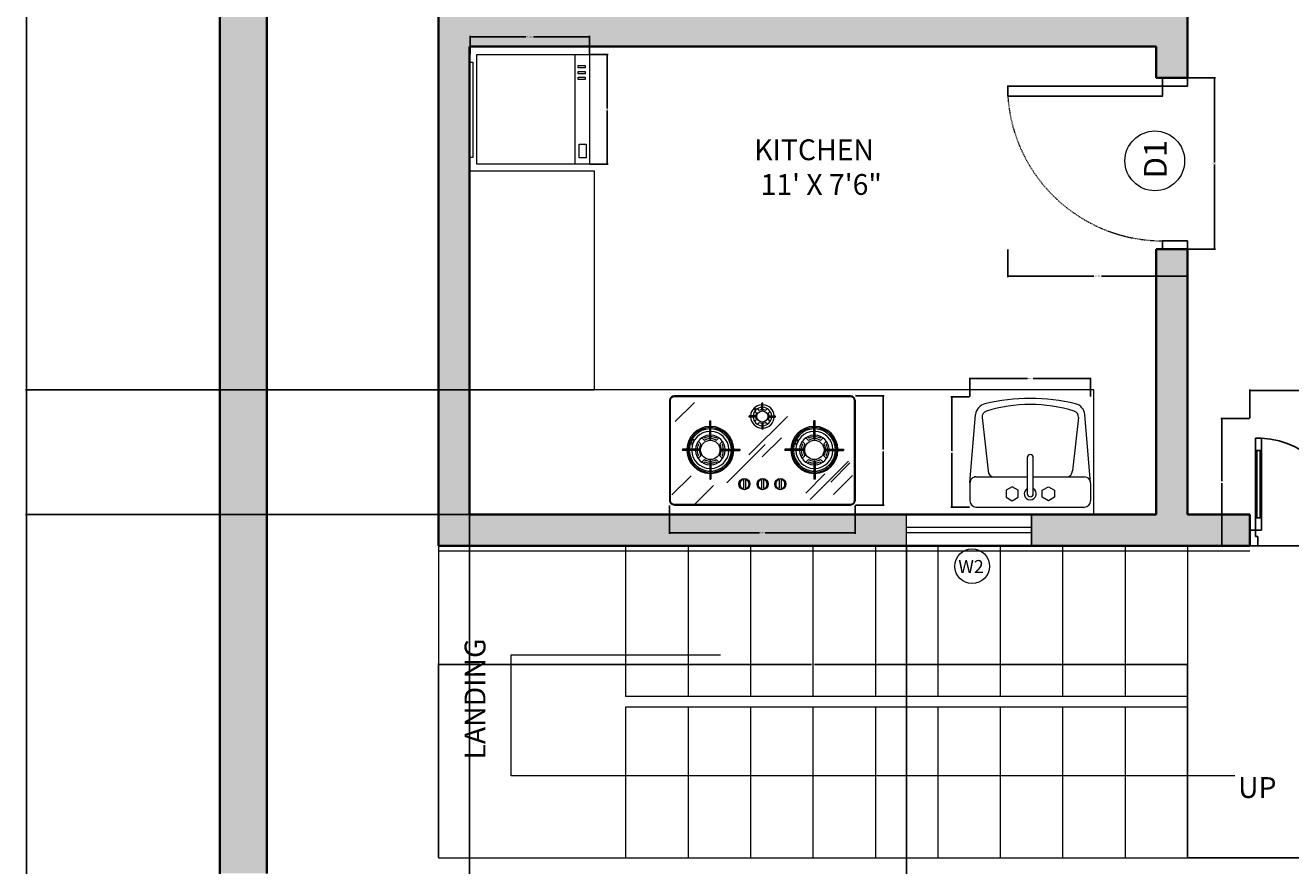
# Model space of a CAD drawing. Units: inches. Extents: x 2701 to 6846, y 811 to 2447.
# Tile 2 of 20: x 2701 to 2944, y 969 to 1130. Entities that reach past the tile are written whole.
import ezdxf

# ---------------------------------------------------------------- set-up
doc = ezdxf.new("R2010")
doc.units = ezdxf.units.IN
doc.linetypes.add('HIDDEN4', pattern=[0.09375, 0.0625, -0.03125])
for name, color, linetype, lineweight in [('A-ANNO-DIMS', 2, 'Continuous', 18), ('A-ANNO-IDEN', 7, 'Continuous', 13), ('A-ANNO-TEXT', 7, 'Continuous', 18), ('A-AREA-IDEN', 7, 'Continuous', 18), ('A-DOOR', 4, 'Continuous', 25), ('A-DOOR-SWNG', 4, 'HIDDEN4', 13), ('A-EQPM', 8, 'Continuous', 18), ('A-FLOR-FIXT', 7, 'Continuous', 18), ('A-FLOR-STRS', 7, 'Continuous', 18), ('A-GLAZ', 4, 'Continuous', 18), ('A-WALL', 7, 'Continuous', 35), ('C-PROP', 7, 'Continuous', 35)]:
    doc.layers.add(name, color=color, linetype=linetype, lineweight=lineweight)
doc.layers.add('A-WALL-PATT', color=18, linetype='Continuous', lineweight=13, true_color=0x000000)
doc.layers.add('C-PROP-PATT', color=18, linetype='Continuous', lineweight=13, true_color=0x000000)
doc.styles.get("Standard").update_dxf_attribs({"font": 'arial.ttf'})
doc.dimstyles.get("Standard").update_dxf_attribs({"dimtxt": 0.18, "dimasz": 0.18, "dimexe": 0.18, "dimexo": 0.0625, "dimgap": 0.09, "dimtad": 0, "dimtih": 1, "dimtoh": 1, "dimdec": 4, "dimzin": 0, "dimdsep": 46, "dimtxsty": 'Standard', "dimcen": 0.09, "dimadec": 0, "dimazin": 0, "dimtfac": 1, "dimtdec": 4, "dimtofl": 0, "dimtmove": 0, "dimatfit": 3, "dimfxl": 1, "dimtolj": 1, "dimtzin": 0, "dimarcsym": 0})

# ---------------------------------------------------------------- blocks, each defined once
blk = doc.blocks.new('A$C09A905BE')
for p, q in [((35, 690), (35, 610)), ((75, 690), (35, 690)), ((75, 610), (75, 690)), ((1125, 690), (1125, 610)), ((1165, 690), (1125, 690)), ((1165, 610), (1165, 690)), ((35, 610), (75, 610)), ((35, 180), (35, 610)), ((35, 610), (75, 610)), ((45, 180), (45, 610)), ((45, 610), (65, 610)), ((65, 610), (65, 180)), ((75, 610), (75, 180)), ((1125, 610), (1165, 610)), ((1125, 180), (1125, 610)), ((1125, 610), (1165, 610)), ((1135, 180), (1135, 610)), ((1135, 610), (1155, 610)), ((1155, 610), (1155, 180)), ((1165, 610), (1165, 180)), ((35, 100), (35, 180)), ((35, 180), (75, 180)), ((75, 180), (35, 180)), ((65, 180), (45, 180)), ((75, 180), (75, 100)), ((1125, 100), (1125, 180)), ((1125, 180), (1165, 180)), ((1165, 180), (1125, 180)), ((1155, 180), (1135, 180)), ((1165, 180), (1165, 100)), ((0, 0), (0, 100)), ((0, 100), (35, 100)), ((35, 100), (35, 60)), ((75, 100), (35, 100)), ((1165, 100), (1125, 100)), ((1165, 100), (1200, 100)), ((1165, 60), (1165, 100)), ((1200, 100), (1200, 0)), ((35, 60), (50, 60)), ((50, 60), (50, 50)), ((50, 50), (50, 0)), ((1150, 50), (1150, 60)), ((1150, 60), (1165, 60)), ((1150, 0), (1150, 50)), ((50, 0), (0, 0)), ((1200, 0), (1150, 0))]:
    blk.add_line(p, q)
for centre, start, end in [((42.5, 132.5), 356.66366, 86.66366), ((1157.5, 132.5), 93.33634, 183.33634)]:
    blk.add_arc(centre, 558.4, start, end)
blk = doc.blocks.new('MAIN DOOR')
blk.add_circle((3420.7, 1223.43), 3.42)
at = {"xscale": 0.03, "yscale": 0.03, "zscale": 0.03}
blk.add_blockref('A$C09A905BE', (3402.65, 1202.37), dxfattribs=at)
at = {"insert": (3418.39, 1224.62), "char_height": 2.5, "attachment_point": 1}
blk.add_mtext('MD', dxfattribs=at)
blk = doc.blocks.new('A$C301E58BA')
for p, q in [((0, 0.3491), (0, 0.4241)), ((0.475, 0.4491), (0.025, 0.4491)), ((0.15, 0.4085), (0.175, 0.423)), ((0.175, 0.423), (0.2, 0.4085)), ((0.325, 0.423), (0.3, 0.4085)), ((0.35, 0.4085), (0.325, 0.423)), ((0.5, 0.3491), (0.5, 0.4241)), ((0.15, 0.3797), (0.15, 0.4085)), ((0.175, 0.3652), (0.15, 0.3797)), ((0.2, 0.3797), (0.175, 0.3652)), ((0.2, 0.4085), (0.2, 0.3797)), ((0.2375, 0.3941), (0.2375, 0.2441)), ((0.2625, 0.2441), (0.2625, 0.3941)), ((0.3, 0.4085), (0.3, 0.3797)), ((0.3, 0.3797), (0.325, 0.3652)), ((0.325, 0.3652), (0.35, 0.3797)), ((0.35, 0.3797), (0.35, 0.4085)), ((0, 0.3491), (0.0236, 0.0657)), ((0.2375, 0.3241), (0.025, 0.3241)), ((0.475, 0.3241), (0.2625, 0.3241)), ((0.5, 0.3491), (0.4764, 0.0657)), ((0.0504, 0.0779), (0.075, 0.2991)), ((0.4496, 0.0779), (0.425, 0.2991))]:
    blk.add_line(p, q)
for centre, radius, start, end in [((0.025, 0.4241), 0.025, 90, 180), ((0.475, 0.4241), 0.025, 0, 90), ((0.25, 0.3941), 0.025, 300, 240), ((0.25, 0.3941), 0.0125, 0, 180), ((0.025, 0.3491), 0.025, 180, 270), ((0.1, 0.2991), 0.025, 90, 180), ((0.4, 0.2991), 0.025, 0, 90), ((0.475, 0.3491), 0.025, 270, 0), ((0.25, 0.2441), 0.0125, 180, 0), ((0.0734, 0.0698), 0.05, 184.7636, 256.6119), ((0.0753, 0.0751), 0.025, 173.6598, 253.0688), ((0.4247, 0.0751), 0.025, 286.9312, 6.3402), ((0.4266, 0.0698), 0.05, 283.3881, 355.2364), ((0.25, 0.8116), 0.8125, 256.6119, 283.3881), ((0.25, 0.6491), 0.625, 253.0688, 286.9312)]:
    blk.add_arc(centre, radius, start, end)
blk = doc.blocks.new('A$C038F079D')
for p, q in [((23.9, 336.8), (101.3, 414.2)), ((377.5, 410.6), (372.5, 410.6)), ((320.9, 202.7), (475.7, 357.5)), ((427.1, 359.8), (427.1, 354.8)), ((587.4, 339.9), (582.4, 339.9)), ((377.5, 305.6), (372.5, 305.6)), ((374.2, 193.8), (451.6, 271.2)), ((53.2, 224.7), (53.2, 219.7)), ((232.1, 89.3), (386.9, 244.1)), ((284, 224.7), (284, 219.7)), ((466, 224.7), (466, 219.7)), ((701.8, 224.7), (701.8, 219.7)), ((130.3, 173.3), (141.1, 184.1)), ((137.3, 169), (142.6, 174.2)), ((567.6, 22.2), (722.4, 177)), ((650.5, 92.2), (727.9, 169.6)), ((10.1, 41), (87.5, 118.4)), ((549.9, 47.9), (627.2, 125.3)), ((587.4, 103.7), (582.4, 103.7)), ((661.4, 42), (738.7, 119.3)), ((100.9, 1.5), (178.3, 78.9))]:
    blk.add_line(p, q)
at = {"ltscale": 0.18}
for p, q in [((372.5, 384.7), (372.5, 410.6)), ((377.5, 384.7), (377.5, 410.6)), ((322.3, 354.8), (322.3, 359.8)), ((347.6, 359.8), (322.3, 359.8)), ((350.8, 370.2), (343.5, 377.5)), ((362.2, 381.5), (354.8, 388.8)), ((387.8, 381.5), (395.2, 388.8)), ((399.2, 370.2), (406.5, 377.5)), ((402.4, 359.8), (427.1, 359.8)), ((162.6, 339.9), (167.6, 339.9)), ((162.6, 267.1), (162.6, 339.9)), ((167.6, 267.1), (167.6, 339.9)), ((347.6, 354.8), (322.3, 354.8)), ((343.5, 337.2), (350.8, 344.5)), ((354.8, 325.8), (362.2, 333.1)), ((372.5, 329.9), (372.5, 305.6)), ((377.5, 329.9), (377.5, 305.6)), ((395.2, 325.8), (387.8, 333.1)), ((406.5, 337.2), (399.2, 344.5)), ((402.4, 354.8), (427.1, 354.8)), ((582.4, 267.1), (582.4, 339.9)), ((587.4, 267.1), (587.4, 339.9)), ((116.2, 257), (127, 246.2)), ((130.3, 271.1), (141.1, 260.3)), ((137.3, 275.4), (142.6, 270.2)), ((187.6, 270.2), (192.8, 275.4)), ((189, 260.3), (199.8, 271.1)), ((203.2, 246.2), (214, 257)), ((546.8, 246.2), (536, 257)), ((561, 260.3), (550.2, 271.1)), ((562.4, 270.2), (557.2, 275.4)), ((612.7, 275.4), (607.4, 270.2)), ((619.7, 271.1), (608.9, 260.3)), ((633.8, 257), (623, 246.2)), ((125.1, 224.7), (53.2, 224.7)), ((125.1, 219.7), (53.2, 219.7)), ((111.9, 250), (117.1, 244.7)), ((210, 224.7), (284, 224.7)), ((210, 219.7), (284, 219.7)), ((213.1, 244.7), (218.3, 250)), ((540, 224.7), (466, 224.7)), ((540, 219.7), (466, 219.7)), ((536.9, 244.7), (531.7, 250)), ((629.9, 224.7), (701.8, 224.7)), ((629.9, 219.7), (701.8, 219.7)), ((638.1, 250), (632.9, 244.7)), ((111.9, 194.5), (117.1, 199.7)), ((116.2, 187.5), (127, 198.3)), ((162.6, 177.3), (162.6, 103.7)), ((167.6, 177.3), (167.6, 103.7)), ((187.6, 174.2), (192.8, 169)), ((189, 184.1), (199.8, 173.3)), ((203.2, 198.3), (214, 187.5)), ((213.1, 199.7), (218.3, 194.5)), ((536.9, 199.7), (531.7, 194.5)), ((546.8, 198.3), (536, 187.5)), ((561, 184.1), (550.2, 173.3)), ((562.4, 174.2), (557.2, 169)), ((582.4, 177.3), (582.4, 103.7)), ((587.4, 177.3), (587.4, 103.7)), ((612.7, 169), (607.4, 174.2)), ((619.7, 173.3), (608.9, 184.1)), ((633.8, 187.5), (623, 198.3)), ((638.1, 194.5), (632.9, 199.7)), ((162.6, 103.7), (167.6, 103.7)), ((298.6, 99.8), (298.6, 69)), ((306.6, 99.8), (306.6, 69)), ((372, 99.8), (372, 69)), ((380, 99.8), (380, 69)), ((443.4, 99.8), (443.4, 69)), ((451.4, 99.8), (451.4, 69))]:
    blk.add_line(p, q, dxfattribs=at)
for points in [[(20, 0), (730, 0, 0.414214), (750, 20), (750, 420, 0.414214), (730, 440), (20, 440, 0.414214), (0, 420), (0, 20, 0.414214)], [(20, 3), (730, 3, 0.414214), (747, 20), (747, 420, 0.414214), (730, 437), (20, 437, 0.414214), (3, 420), (3, 20, 0.414214)]]:
    blk.add_lwpolyline(points, format="xyb", close=True)
for centre in [(345.9, 386.3), (94.7, 261.5), (514.6, 260.8), (89.1, 248.3), (509, 247.6)]:
    blk.add_circle(centre, 3.73)
for centre, radius in [((375, 357.3), 22.4), ((165.1, 222.2), 39), ((584.9, 222.2), 39), ((302.6, 84.4), 22.5), ((302.6, 84.4), 21.5), ((376, 84.4), 22.5), ((376, 84.4), 21.5), ((447.4, 84.4), 22.5), ((447.4, 84.4), 21.5)]:
    blk.add_circle(centre, radius, dxfattribs=at)
for centre, radius, start, end in [((375, 357.3), 47.4, 93.0255, 176.9745), ((375, 357.3), 37.4, 93.8363, 176.1637), ((346.8, 357.3), 2.62, 287.6318, 72.3682), ((375, 357.3), 27.4, 151.9979, 174.8384), ((375, 357.3), 27.4, 95.203, 118.0021), ((375, 385), 2.52, 187.9505, 352.0495), ((375, 357.3), 47.4, 3.0255, 86.9745), ((375, 357.3), 37.4, 3.8363, 86.1637), ((375, 357.3), 27.4, 61.9979, 84.797), ((375, 357.3), 27.4, 5.206, 28.0021), ((402.7, 357.3), 2.52, 97.2236, 262.7764), ((165.1, 222.2), 95, 91.5918, 178.4082), ((165.1, 222.2), 90, 91.5918, 178.4082), ((165.1, 222.2), 85, 91.6854, 178.3146), ((165.1, 222.2), 90, 1.5918, 88.4082), ((165.1, 222.2), 85, 1.6854, 88.3146), ((165.1, 222.2), 95, 1.5918, 88.4082), ((375, 357.3), 47.4, 183.0255, 266.9745), ((375, 357.3), 37.4, 183.8363, 266.1637), ((375, 357.3), 27.4, 185.1616, 208.0021), ((375, 357.3), 27.4, 241.9979, 264.7569), ((375, 330), 2.5, 358.3317, 181.6683), ((375, 357.3), 47.4, 273.0255, 356.9745), ((375, 357.3), 37.4, 273.8363, 356.1637), ((375, 357.3), 27.4, 275.2431, 298.0021), ((375, 357.3), 27.4, 331.9979, 354.794), ((584.9, 222.2), 95, 91.5918, 178.4082), ((584.9, 222.2), 90, 91.5918, 178.4082), ((584.9, 222.2), 85, 91.6854, 178.3146), ((584.9, 222.2), 90, 1.5918, 88.4082), ((584.9, 222.2), 85, 1.6854, 88.3146), ((584.9, 222.2), 95, 1.5918, 88.4082), ((165.1, 222.2), 75, 91.9102, 178.0898), ((165.1, 222.2), 60, 92.388, 177.612), ((165.1, 222.2), 45, 93.1847, 122.1604), ((165.1, 222.2), 53, 92.7036, 115.1461), ((165.1, 267.4), 2.52, 186.7354, 353.2646), ((165.1, 222.2), 75, 1.9102, 88.0898), ((165.1, 222.2), 60, 2.388, 87.612), ((165.1, 222.2), 53, 64.8539, 87.2964), ((165.1, 222.2), 45, 57.8396, 86.8153), ((584.9, 222.2), 75, 91.9102, 178.0898), ((584.9, 222.2), 60, 92.388, 177.612), ((584.9, 222.2), 45, 93.1847, 122.1604), ((584.9, 222.2), 53, 92.7036, 115.1461), ((584.9, 267.3), 2.51, 183.9579, 356.0421), ((584.9, 222.2), 75, 1.9102, 88.0898), ((584.9, 222.2), 60, 2.388, 87.612), ((584.9, 222.2), 53, 64.8539, 87.2964), ((584.9, 222.2), 45, 57.8396, 86.8153), ((165.1, 222.2), 95, 181.5918, 268.4082), ((165.1, 222.2), 90, 181.5918, 268.4082), ((165.1, 222.2), 85, 181.6854, 268.3146), ((165.1, 222.2), 75, 181.9102, 268.0898), ((165.1, 222.2), 60, 182.388, 267.612), ((165.1, 222.2), 53, 154.8539, 177.2964), ((165.1, 222.2), 53, 182.7036, 205.1461), ((165.1, 222.2), 45, 147.8396, 176.8153), ((119.3, 222.2), 2.64, 288.751, 71.249), ((165.1, 222.2), 45, 183.1847, 212.1604), ((165.1, 222.2), 75, 271.9102, 358.0898), ((165.1, 222.2), 60, 272.388, 357.612), ((165.1, 222.2), 85, 271.6854, 358.3146), ((165.1, 222.2), 90, 271.5918, 358.4082), ((165.1, 222.2), 95, 271.5918, 358.4082), ((165.1, 222.2), 45, 3.1847, 32.1604), ((165.1, 222.2), 45, 327.8396, 356.8153), ((210.9, 222.2), 2.67, 110.5507, 249.4493), ((165.1, 222.2), 53, 2.7036, 25.1461), ((165.1, 222.2), 53, 334.8539, 357.2964), ((584.9, 222.2), 95, 181.5918, 268.4082), ((584.9, 222.2), 90, 181.5918, 268.4082), ((584.9, 222.2), 85, 181.6854, 268.3146), ((584.9, 222.2), 75, 181.9102, 268.0898), ((584.9, 222.2), 60, 182.388, 267.612), ((584.9, 222.2), 53, 154.8539, 177.2964), ((584.9, 222.2), 53, 182.7036, 205.1461), ((584.9, 222.2), 45, 147.8396, 176.8153), ((539.2, 222.2), 2.63, 288.412, 71.588), ((584.9, 222.2), 45, 183.1847, 212.1604), ((584.9, 222.2), 90, 271.5918, 358.4082), ((584.9, 222.2), 85, 271.6854, 358.3146), ((584.9, 222.2), 75, 271.9102, 358.0898), ((584.9, 222.2), 60, 272.388, 357.612), ((584.9, 222.2), 95, 271.5918, 358.4082), ((584.9, 222.2), 45, 3.1847, 32.1604), ((584.9, 222.2), 45, 327.8396, 356.8153), ((630.5, 222.2), 2.58, 104.2945, 255.7055), ((584.9, 222.2), 53, 2.7036, 25.1461), ((584.9, 222.2), 53, 334.8539, 357.2964), ((165.1, 222.2), 45, 237.8396, 266.8153), ((165.1, 222.2), 53, 244.8539, 267.2964), ((165.1, 222.2), 45, 273.1847, 302.1604), ((165.1, 222.2), 53, 272.7036, 295.1461), ((584.9, 222.2), 45, 237.8396, 266.8153), ((584.9, 222.2), 53, 244.8539, 267.2964), ((584.9, 176.5), 2.63, 17.9418, 162.0582), ((584.9, 222.2), 45, 273.1847, 302.1604), ((584.9, 222.2), 53, 272.7036, 295.1461), ((302.6, 84.4), 18.5, 111.3237, 248.6763), ((296.6, 99.8), 2, 0, 111.3237), ((296.6, 69), 2, 248.6763, 0), ((308.6, 99.8), 2, 68.6763, 180), ((308.6, 69), 2, 180, 291.3237), ((302.6, 84.4), 18.5, 291.3237, 68.6763), ((376, 84.4), 18.5, 111.3237, 248.6763), ((370, 99.8), 2, 0, 111.3237), ((370, 69), 2, 248.6763, 0), ((382, 99.8), 2, 68.6763, 180), ((382, 69), 2, 180, 291.3237), ((376, 84.4), 18.5, 291.3237, 68.6763), ((447.4, 84.4), 18.5, 111.3237, 248.6763), ((441.4, 99.8), 2, 0, 111.3237), ((441.4, 69), 2, 248.6763, 0), ((453.4, 99.8), 2, 68.6763, 180), ((453.4, 69), 2, 180, 291.3237), ((447.4, 84.4), 18.5, 291.3237, 68.6763)]:
    blk.add_arc(centre, radius, start, end, dxfattribs=at)
blk.add_arc((165.1, 176.3), 2.69, 21.7885, 158.2115)
blk = doc.blocks.new('A$C45054F6D')
for p, q in [((33.6, 610), (522.2, 610)), ((33.6, 596), (33.6, 610)), ((522.2, 596), (33.6, 596)), ((522.2, 610), (522.2, 596)), ((0, 575.1), (560, 575.1)), ((0, 0), (0, 575.1)), ((560, 575.1), (560, 0)), ((560, 75), (0, 75)), ((33.3, 53), (103.3, 53)), ((33.3, 16.3), (33.3, 53)), ((103.3, 16.3), (33.3, 16.3)), ((103.3, 53), (103.3, 16.3)), ((432.3, 21.5), (432.3, 58.3)), ((432.3, 58.3), (444.6, 58.3)), ((444.6, 21.5), (432.3, 21.5)), ((444.6, 58.3), (444.6, 21.5)), ((462.1, 21.5), (462.1, 58.3)), ((462.1, 58.3), (474.3, 58.3)), ((474.3, 21.5), (462.1, 21.5)), ((474.3, 58.3), (474.3, 21.5)), ((491.8, 21.5), (491.8, 58.3)), ((491.8, 58.3), (504.1, 58.3)), ((504.1, 21.5), (491.8, 21.5)), ((504.1, 58.3), (504.1, 21.5)), ((560, 0), (0, 0))]:
    blk.add_line(p, q)
blk = doc.blocks.new('DOOR-D1-33IN-PANEL-FRAME')
blk.add_lwpolyline([(0, 33), (0, 31.37), (4.8, 31.37), (4.8, 33), (0, 33)], close=True)
for points in [[(4.32, 33), (0.48, 33)], [(4.8, 0), (4.8, 3.55), (34.54, 3.55), (34.54, 1.63), (0, 1.63), (0, 0)], [(0, 0), (4.8, 0)], [(4.32, 0), (0.48, 0)]]:
    blk.add_lwpolyline(points)
blk = doc.blocks.new('WIN-W2-24IN')
for p, q in [((24, 6), (0, 6)), ((24, 6), (0, 6)), ((0, 0), (0, 6)), ((24, 6), (24, 6)), ((24, 6), (24, 0)), ((24, 3.5), (0, 3.5)), ((24, 2.5), (0, 2.5)), ((24, 0), (0, 0))]:
    blk.add_line(p, q)
blk = doc.blocks.new('*D27')
at = {"layer": 'A-ANNO-DIMS', "color": 0, "lineweight": -2, "transparency": 16777216}
for p, q in [((2889.43, 1086.99), (2889.43, 1081.69)), ((2923.97, 1086.99), (2923.97, 1081.69)), ((2889.61, 1081.87), (2905.98, 1081.87)), ((2923.79, 1081.87), (2907.42, 1081.87))]:
    blk.add_line(p, q, dxfattribs=at)
at = {"layer": 'A-ANNO-DIMS', "color": 0, "transparency": 16777216}
for points in [[(2889.61, 1081.9), (2889.61, 1081.84), (2889.43, 1081.87)], [(2923.79, 1081.9), (2923.79, 1081.84), (2923.97, 1081.87)]]:
    blk.add_solid(points, dxfattribs=at)
at = {"layer": 'Defpoints', "color": 0, "transparency": 16777216}
for p in [(2889.43, 1087.05), (2923.97, 1087.05), (2889.43, 1081.87)]:
    blk.add_point(p, dxfattribs=at)
at = {"layer": 'A-ANNO-DIMS', "color": 0, "transparency": 16777216, "insert": (2906.7, 1081.87), "char_height": 0.18, "attachment_point": 5}
blk.add_mtext('\\A1;D1 35 TYP.', dxfattribs=at)
blk = doc.blocks.new('*D28')
at = {"layer": 'A-ANNO-DIMS', "color": 0, "lineweight": -2, "transparency": 16777216}
for p, q in [((2924.03, 1120.05), (2929.33, 1120.05)), ((2929.15, 1119.87), (2929.15, 1103.73)), ((2929.15, 1087.23), (2929.15, 1103.37)), ((2924.03, 1087.05), (2929.33, 1087.05))]:
    blk.add_line(p, q, dxfattribs=at)
at = {"layer": 'A-ANNO-DIMS', "color": 0, "transparency": 16777216}
for points in [[(2929.12, 1119.87), (2929.18, 1119.87), (2929.15, 1120.05)], [(2929.12, 1087.23), (2929.18, 1087.23), (2929.15, 1087.05)]]:
    blk.add_solid(points, dxfattribs=at)
at = {"layer": 'Defpoints', "color": 0, "transparency": 16777216}
for p in [(2923.97, 1120.05), (2923.97, 1087.05), (2929.15, 1087.05)]:
    blk.add_point(p, dxfattribs=at)
at = {"layer": 'A-ANNO-DIMS', "color": 0, "transparency": 16777216, "insert": (2929.15, 1103.55), "char_height": 0.18, "attachment_point": 5}
blk.add_mtext('\\A1;33 TYP.', dxfattribs=at)
blk = doc.blocks.new('*D31')
at = {"layer": 'A-ANNO-DIMS', "color": 0, "lineweight": -2, "transparency": 16777216}
for p, q in [((2935.97, 1054.6), (2935.97, 1060.11)), ((2936.15, 1059.93), (2952.88, 1059.93)), ((2971.79, 1059.93), (2955.06, 1059.93)), ((2971.97, 1054.6), (2971.97, 1060.11))]:
    blk.add_line(p, q, dxfattribs=at)
at = {"layer": 'A-ANNO-DIMS', "color": 0, "transparency": 16777216}
for points in [[(2936.15, 1059.96), (2936.15, 1059.9), (2935.97, 1059.93)], [(2971.79, 1059.96), (2971.79, 1059.9), (2971.97, 1059.93)]]:
    blk.add_solid(points, dxfattribs=at)
at = {"layer": 'Defpoints', "color": 0, "transparency": 16777216}
for p in [(2971.97, 1059.93), (2935.97, 1054.53), (2971.97, 1054.53)]:
    blk.add_point(p, dxfattribs=at)
at = {"layer": 'A-ANNO-DIMS', "color": 0, "transparency": 16777216, "insert": (2953.97, 1059.93), "char_height": 0.18, "attachment_point": 5}
blk.add_mtext('\\A1;ENTRY DOOR 36', dxfattribs=at)
blk = doc.blocks.new('*D32')
at = {"layer": 'A-ANNO-DIMS', "color": 0, "lineweight": -2, "transparency": 16777216}
for p, q in [((2935.91, 1054.53), (2930.39, 1054.53)), ((2930.57, 1054.35), (2930.57, 1042.47)), ((2930.57, 1030.23), (2930.57, 1042.11)), ((2935.91, 1030.05), (2930.39, 1030.05))]:
    blk.add_line(p, q, dxfattribs=at)
at = {"layer": 'A-ANNO-DIMS', "color": 0, "transparency": 16777216}
for points in [[(2930.54, 1054.35), (2930.6, 1054.35), (2930.57, 1054.53)], [(2930.54, 1030.23), (2930.6, 1030.23), (2930.57, 1030.05)]]:
    blk.add_solid(points, dxfattribs=at)
at = {"layer": 'Defpoints', "color": 0, "transparency": 16777216}
for p in [(2930.57, 1054.53), (2935.97, 1054.53), (2935.97, 1030.05)]:
    blk.add_point(p, dxfattribs=at)
at = {"layer": 'A-ANNO-DIMS', "color": 0, "transparency": 16777216, "insert": (2930.57, 1042.29), "char_height": 0.18, "attachment_point": 5}
blk.add_mtext('\\A1;24', dxfattribs=at)
blk = doc.blocks.new('*D55')
at = {"layer": 'A-ANNO-DIMS', "color": 0, "lineweight": -2, "transparency": 16777216}
for p, q in [((2882.15, 1058.77), (2882.15, 1062.37)), ((2882.33, 1062.19), (2893.2, 1062.19)), ((2905.16, 1062.19), (2894.29, 1062.19)), ((2905.34, 1058.77), (2905.34, 1062.37))]:
    blk.add_line(p, q, dxfattribs=at)
at = {"layer": 'A-ANNO-DIMS', "color": 0, "transparency": 16777216}
for points in [[(2882.33, 1062.22), (2882.33, 1062.16), (2882.15, 1062.19)], [(2905.16, 1062.22), (2905.16, 1062.16), (2905.34, 1062.19)]]:
    blk.add_solid(points, dxfattribs=at)
at = {"layer": 'Defpoints', "color": 0, "transparency": 16777216}
for p in [(2882.15, 1062.19), (2882.15, 1058.71), (2905.34, 1058.71)]:
    blk.add_point(p, dxfattribs=at)
at = {"layer": 'A-ANNO-DIMS', "color": 0, "transparency": 16777216, "insert": (2893.74, 1062.19), "char_height": 0.18, "attachment_point": 5}
blk.add_mtext('\\A1;SINK 23', dxfattribs=at)
blk = doc.blocks.new('*D56')
at = {"layer": 'A-ANNO-DIMS', "color": 0, "lineweight": -2, "transparency": 16777216}
for p, q in [((2882.09, 1058.71), (2878.5, 1058.71)), ((2878.68, 1058.53), (2878.68, 1048.29)), ((2878.68, 1037.68), (2878.68, 1047.93)), ((2882.09, 1037.5), (2878.5, 1037.5))]:
    blk.add_line(p, q, dxfattribs=at)
at = {"layer": 'A-ANNO-DIMS', "color": 0, "transparency": 16777216}
for points in [[(2878.65, 1058.53), (2878.71, 1058.53), (2878.68, 1058.71)], [(2878.65, 1037.68), (2878.71, 1037.68), (2878.68, 1037.5)]]:
    blk.add_solid(points, dxfattribs=at)
at = {"layer": 'Defpoints', "color": 0, "transparency": 16777216}
for p in [(2882.15, 1058.71), (2878.68, 1037.5), (2882.15, 1037.5)]:
    blk.add_point(p, dxfattribs=at)
at = {"layer": 'A-ANNO-DIMS', "color": 0, "transparency": 16777216, "insert": (2878.68, 1048.11), "char_height": 0.18, "attachment_point": 5}
blk.add_mtext('\\A1;21', dxfattribs=at)
blk = doc.blocks.new('*D57')
at = {"layer": 'A-ANNO-DIMS', "color": 0, "lineweight": -2, "transparency": 16777216}
for p, q in [((2824.38, 1037.83), (2824.38, 1032.35)), ((2860.12, 1037.83), (2860.12, 1032.35)), ((2824.56, 1032.53), (2841.73, 1032.53)), ((2859.94, 1032.53), (2842.77, 1032.53))]:
    blk.add_line(p, q, dxfattribs=at)
at = {"layer": 'A-ANNO-DIMS', "color": 0, "transparency": 16777216}
for points in [[(2824.56, 1032.56), (2824.56, 1032.5), (2824.38, 1032.53)], [(2859.94, 1032.56), (2859.94, 1032.5), (2860.12, 1032.53)]]:
    blk.add_solid(points, dxfattribs=at)
at = {"layer": 'Defpoints', "color": 0, "transparency": 16777216}
for p in [(2824.38, 1037.89), (2860.12, 1037.89), (2860.12, 1032.53)]:
    blk.add_point(p, dxfattribs=at)
at = {"layer": 'A-ANNO-DIMS', "color": 0, "transparency": 16777216, "insert": (2842.25, 1032.53), "char_height": 0.18, "attachment_point": 5}
blk.add_mtext('\\A1;HOB 36', dxfattribs=at)
blk = doc.blocks.new('*D58')
at = {"layer": 'A-ANNO-DIMS', "color": 0, "lineweight": -2, "transparency": 16777216}
for p, q in [((2860.18, 1058.86), (2865.66, 1058.86)), ((2865.48, 1058.68), (2865.48, 1048.55)), ((2865.48, 1038.07), (2865.48, 1048.19)), ((2860.18, 1037.89), (2865.66, 1037.89))]:
    blk.add_line(p, q, dxfattribs=at)
at = {"layer": 'A-ANNO-DIMS', "color": 0, "transparency": 16777216}
for points in [[(2865.45, 1058.68), (2865.51, 1058.68), (2865.48, 1058.86)], [(2865.45, 1038.07), (2865.51, 1038.07), (2865.48, 1037.89)]]:
    blk.add_solid(points, dxfattribs=at)
at = {"layer": 'Defpoints', "color": 0, "transparency": 16777216}
for p in [(2860.12, 1058.86), (2865.48, 1058.86), (2860.12, 1037.89)]:
    blk.add_point(p, dxfattribs=at)
at = {"layer": 'A-ANNO-DIMS', "color": 0, "transparency": 16777216, "insert": (2865.48, 1048.37), "char_height": 0.18, "attachment_point": 5}
blk.add_mtext('\\A1;21', dxfattribs=at)
blk = doc.blocks.new('*D59')
at = {"layer": 'A-ANNO-DIMS', "color": 0, "lineweight": -2, "transparency": 16777216}
for p, q in [((2786.06, 1124.54), (2786.06, 1128.1)), ((2786.24, 1127.92), (2796.81, 1127.92)), ((2808.83, 1127.92), (2798.26, 1127.92)), ((2809.01, 1124.54), (2809.01, 1128.1))]:
    blk.add_line(p, q, dxfattribs=at)
at = {"layer": 'A-ANNO-DIMS', "color": 0, "transparency": 16777216}
for points in [[(2786.24, 1127.95), (2786.24, 1127.89), (2786.06, 1127.92)], [(2808.83, 1127.95), (2808.83, 1127.89), (2809.01, 1127.92)]]:
    blk.add_solid(points, dxfattribs=at)
at = {"layer": 'Defpoints', "color": 0, "transparency": 16777216}
for p in [(2786.06, 1127.92), (2786.06, 1124.48), (2809.01, 1124.48)]:
    blk.add_point(p, dxfattribs=at)
at = {"layer": 'A-ANNO-DIMS', "color": 0, "transparency": 16777216, "insert": (2797.53, 1127.92), "char_height": 0.18, "attachment_point": 5}
blk.add_mtext('\\A1;FRIDGE 23', dxfattribs=at)
blk = doc.blocks.new('*D60')
at = {"layer": 'A-ANNO-DIMS', "color": 0, "lineweight": -2, "transparency": 16777216}
for p, q in [((2809.07, 1124.48), (2812.63, 1124.48)), ((2812.45, 1124.3), (2812.45, 1114.12)), ((2812.45, 1103.59), (2812.45, 1113.76)), ((2809.07, 1103.41), (2812.63, 1103.41))]:
    blk.add_line(p, q, dxfattribs=at)
at = {"layer": 'A-ANNO-DIMS', "color": 0, "transparency": 16777216}
for points in [[(2812.42, 1124.3), (2812.48, 1124.3), (2812.45, 1124.48)], [(2812.42, 1103.59), (2812.48, 1103.59), (2812.45, 1103.41)]]:
    blk.add_solid(points, dxfattribs=at)
at = {"layer": 'Defpoints', "color": 0, "transparency": 16777216}
for p in [(2809.01, 1124.48), (2812.45, 1124.48), (2809.01, 1103.41)]:
    blk.add_point(p, dxfattribs=at)
at = {"layer": 'A-ANNO-DIMS', "color": 0, "transparency": 16777216, "insert": (2812.45, 1113.94), "char_height": 0.18, "attachment_point": 5}
blk.add_mtext('\\A1;21', dxfattribs=at)
blk = doc.blocks.new('*D66')
at = {"layer": 'A-ANNO-DIMS', "color": 0, "lineweight": -2, "transparency": 16777216}
for p, q in [((2737.91, 1504.05), (2700.59, 1504.05)), ((2700.77, 1503.87), (2700.77, 1180.23)), ((2700.77, 856.23), (2700.77, 1179.87)), ((2737.91, 856.05), (2700.59, 856.05))]:
    blk.add_line(p, q, dxfattribs=at)
at = {"layer": 'A-ANNO-DIMS', "color": 0, "transparency": 16777216}
for points in [[(2700.74, 1503.87), (2700.8, 1503.87), (2700.77, 1504.05)], [(2700.74, 856.23), (2700.8, 856.23), (2700.77, 856.05)]]:
    blk.add_solid(points, dxfattribs=at)
at = {"layer": 'Defpoints', "color": 0, "transparency": 16777216}
for p in [(2700.77, 1504.05), (2737.97, 1504.05), (2737.97, 856.05)]:
    blk.add_point(p, dxfattribs=at)
at = {"layer": 'A-ANNO-DIMS', "color": 0, "transparency": 16777216, "insert": (2700.77, 1180.05), "char_height": 0.18, "attachment_point": 5}
blk.add_mtext('\\A1;648', dxfattribs=at)
blk = doc.blocks.new('*D73')
at = {"layer": 'A-ANNO-DIMS', "color": 0, "lineweight": -2, "transparency": 16777216}
for p, q in [((2809.91, 1060.05), (2700.59, 1060.05)), ((2700.77, 1059.87), (2700.77, 1048.23)), ((2700.77, 1036.23), (2700.77, 1047.87)), ((2785.91, 1036.05), (2700.59, 1036.05))]:
    blk.add_line(p, q, dxfattribs=at)
at = {"layer": 'A-ANNO-DIMS', "color": 0, "transparency": 16777216}
for points in [[(2700.74, 1059.87), (2700.8, 1059.87), (2700.77, 1060.05)], [(2700.74, 1036.23), (2700.8, 1036.23), (2700.77, 1036.05)]]:
    blk.add_solid(points, dxfattribs=at)
at = {"layer": 'Defpoints', "color": 0, "transparency": 16777216}
for p in [(2700.77, 1060.05), (2809.97, 1060.05), (2785.97, 1036.05)]:
    blk.add_point(p, dxfattribs=at)
at = {"layer": 'A-ANNO-DIMS', "color": 0, "transparency": 16777216, "insert": (2700.77, 1048.05), "char_height": 0.18, "attachment_point": 5}
blk.add_mtext('\\A1;24', dxfattribs=at)
blk = doc.blocks.new('*D74')
at = {"layer": 'A-ANNO-DIMS', "color": 0, "lineweight": -2, "transparency": 16777216}
for p, q in [((2785.97, 1035.99), (2785.97, 818.67)), ((2869.97, 1029.99), (2869.97, 818.67)), ((2786.15, 818.85), (2827.75, 818.85)), ((2869.79, 818.85), (2828.19, 818.85))]:
    blk.add_line(p, q, dxfattribs=at)
at = {"layer": 'A-ANNO-DIMS', "color": 0, "transparency": 16777216}
for points in [[(2786.15, 818.88), (2786.15, 818.82), (2785.97, 818.85)], [(2869.79, 818.88), (2869.79, 818.82), (2869.97, 818.85)]]:
    blk.add_solid(points, dxfattribs=at)
at = {"layer": 'Defpoints', "color": 0, "transparency": 16777216}
for p in [(2785.97, 1036.05), (2869.97, 1030.05), (2869.97, 818.85)]:
    blk.add_point(p, dxfattribs=at)
at = {"layer": 'A-ANNO-DIMS', "color": 0, "transparency": 16777216, "insert": (2827.97, 818.85), "char_height": 0.18, "attachment_point": 5}
blk.add_mtext('\\A1;84', dxfattribs=at)
blk = doc.blocks.new('*D78')
at = {"layer": 'A-ANNO-DIMS', "color": 0, "lineweight": -2, "transparency": 16777216}
for p, q in [((2779.97, 970.11), (2779.97, 1007.43)), ((2780.15, 1007.25), (2851.69, 1007.25)), ((2923.79, 1007.25), (2852.25, 1007.25)), ((2923.97, 970.11), (2923.97, 1007.43))]:
    blk.add_line(p, q, dxfattribs=at)
at = {"layer": 'A-ANNO-DIMS', "color": 0, "transparency": 16777216}
for points in [[(2780.15, 1007.28), (2780.15, 1007.22), (2779.97, 1007.25)], [(2923.79, 1007.28), (2923.79, 1007.22), (2923.97, 1007.25)]]:
    blk.add_solid(points, dxfattribs=at)
at = {"layer": 'Defpoints', "color": 0, "transparency": 16777216}
for p in [(2923.97, 1007.25), (2779.97, 970.05), (2923.97, 970.05)]:
    blk.add_point(p, dxfattribs=at)
at = {"layer": 'A-ANNO-DIMS', "color": 0, "transparency": 16777216, "insert": (2851.97, 1007.25), "char_height": 0.18, "attachment_point": 5}
blk.add_mtext('\\A1;144', dxfattribs=at)
blk = doc.blocks.new('*D79')
at = {"layer": 'A-ANNO-DIMS', "color": 0, "lineweight": -2, "transparency": 16777216}
for p, q in [((2924.03, 1030.05), (2961.35, 1030.05)), ((2961.17, 1029.87), (2961.17, 1000.23)), ((2961.17, 970.23), (2961.17, 999.87)), ((2924.03, 970.05), (2961.35, 970.05))]:
    blk.add_line(p, q, dxfattribs=at)
at = {"layer": 'A-ANNO-DIMS', "color": 0, "transparency": 16777216}
for points in [[(2961.14, 1029.87), (2961.2, 1029.87), (2961.17, 1030.05)], [(2961.14, 970.23), (2961.2, 970.23), (2961.17, 970.05)]]:
    blk.add_solid(points, dxfattribs=at)
at = {"layer": 'Defpoints', "color": 0, "transparency": 16777216}
for p in [(2923.97, 1030.05), (2923.97, 970.05), (2961.17, 970.05)]:
    blk.add_point(p, dxfattribs=at)
at = {"layer": 'A-ANNO-DIMS', "color": 0, "transparency": 16777216, "insert": (2961.17, 1000.05), "char_height": 0.18, "attachment_point": 5}
blk.add_mtext('\\A1;60', dxfattribs=at)

msp = doc.modelspace()

# ---------------------------------------------------------------- hatches: boundary and pattern name
at = {"layer": 'A-WALL-PATT'}
h = msp.add_hatch(color=256, dxfattribs=at)
h.dxf.hatch_style = 1
h.paths.add_polyline_path([(3085.97, 1456.05), (3085.97, 1348.05), (3091.97, 1348.05), (3091.97, 1360.05), (3091.97, 1462.05), (2960.09, 1462.05), (2960.09, 1456.05), (2971.97, 1456.05), (2971.97, 1372.05), (2923.97, 1372.05), (2923.97, 1378.05), (2917.97, 1378.05), (2917.97, 1351.05), (2923.97, 1351.05), (2923.97, 1366.05), (2971.97, 1366.05), (2971.97, 1351.05), (2976.77, 1351.05), (2977.97, 1351.05), (2977.97, 1456.05)])
h.paths.add_polyline_path([(2779.97, 1462.05), (2779.97, 1342.05), (2785.97, 1342.05), (2785.97, 1456.05), (2917.97, 1456.05), (2917.97, 1408.05), (2922.33, 1408.05), (2923.97, 1408.05), (2923.97, 1456.05), (2937.09, 1456.05), (2937.09, 1462.05)])
h.paths.add_polyline_path([(2779.97, 1306.05), (2779.97, 1294.24), (2785.97, 1294.24), (2785.97, 1306.05), (2851.37, 1306.05, -0.025815), (2852.62, 1306.11, -0.025815), (2853.87, 1306.05), (2863.97, 1306.05), (2863.97, 1258.05), (2857.97, 1258.05), (2857.97, 1252.05), (2878.97, 1252.05), (2878.97, 1258.05), (2869.97, 1258.05), (2869.97, 1306.05), (2923.97, 1306.05), (2923.97, 1318.05), (2919.17, 1318.05), (2917.97, 1318.05), (2917.97, 1312.05), (2785.97, 1312.05), (2785.97, 1318.05), (2779.97, 1318.05)])
h.paths.add_polyline_path([(2785.97, 1252.05), (2827.97, 1252.05), (2827.97, 1256.41), (2827.97, 1258.05), (2785.97, 1258.05), (2785.97, 1271.24), (2779.97, 1271.24), (2779.97, 1174.05), (2785.97, 1174.05)])
h.paths.add_polyline_path([(2779.97, 1030.05), (2869.97, 1030.05), (2869.97, 1036.05), (2785.97, 1036.05), (2785.97, 1126.05), (2917.97, 1126.05), (2917.97, 1120.05), (2923.97, 1120.05), (2923.97, 1258.05), (2911.97, 1258.05), (2911.97, 1253.25), (2911.97, 1252.05), (2917.97, 1252.05), (2917.97, 1132.05), (2785.97, 1132.05), (2785.97, 1144.05), (2779.97, 1144.05)])
h.paths.add_polyline_path([(2935.97, 1030.05), (2935.97, 1033.05), (2935.97, 1036.05), (2923.97, 1036.05), (2923.97, 1087.05), (2919.17, 1087.05), (2917.97, 1087.05), (2917.97, 1036.05), (2893.97, 1036.05), (2893.97, 1030.05)])
h.paths.add_polyline_path([(2971.97, 1036.05), (2971.97, 1030.05), (3091.97, 1030.05), (3091.97, 1060.05), (3085.97, 1060.05), (3085.97, 1036.05)])
h.paths.add_polyline_path([(3085.97, 1084.05), (3091.97, 1084.05), (3091.97, 1096.05), (3091.97, 1268.89), (3085.97, 1268.89), (3085.97, 1258.05), (3001.97, 1258.05), (3001.97, 1270.05), (2995.97, 1270.05), (2995.97, 1252.05), (3085.97, 1252.05)])
h.paths.add_polyline_path([(3085.97, 1306.05), (3085.97, 1291.89), (3091.97, 1291.89), (3091.97, 1318.05), (3085.97, 1318.05), (3085.97, 1312.05), (2977.97, 1312.05), (2977.97, 1318.05), (2971.97, 1318.05), (2971.97, 1306.05), (2995.97, 1306.05), (2995.97, 1300.05), (3000.33, 1300.05), (3001.97, 1300.05), (3001.97, 1306.05)])
at = {"layer": 'C-PROP-PATT'}
h = msp.add_hatch(color=256, dxfattribs=at)
h.dxf.hatch_style = 1
h.paths.add_polyline_path([(3145.97, 1504.05), (2737.97, 1504.05), (2737.97, 967.05), (2746.97, 967.05), (2746.97, 1495.05), (3136.97, 1495.05), (3136.97, 865.05), (3130.97, 865.05), (3130.97, 856.05), (3145.97, 856.05)])
h.paths.add_polyline_path([(3070.97, 865.05), (2746.97, 865.05), (2746.97, 871.05), (2737.97, 871.05), (2737.97, 856.05), (3070.97, 856.05)], flags=17)

# ---------------------------------------------------------------- linework, layer by layer
at = {"layer": 'A-ANNO-IDEN'}
for centre, radius in [((2917.69, 1104.06), 5.74), ((2882.58, 1026.12), 3.34)]:
    msp.add_circle(centre, radius, dxfattribs=at)
at = {"layer": 'A-DOOR-SWNG'}
msp.add_arc((2919.17, 1118.49), 29.81, 183.8183, 270, dxfattribs=at)
at = {"layer": 'A-FLOR-FIXT'}
for p, q in [((2809.97, 1102.05), (2785.97, 1102.05)), ((2809.97, 1060.05), (2809.97, 1102.05)), ((2905.97, 1060.05), (2809.97, 1060.05)), ((2905.97, 1036.05), (2905.97, 1060.05))]:
    msp.add_line(p, q, dxfattribs=at)
at = {"layer": 'A-FLOR-STRS'}
for p, q in [((2779.97, 1030.05), (2779.97, 970.05)), ((2935.97, 1029.05), (2779.97, 1029.05)), ((2815.97, 1030.05), (2815.97, 1001.05)), ((2827.97, 1030.05), (2827.97, 1001.05)), ((2839.97, 1030.05), (2839.97, 1001.05)), ((2851.97, 1030.05), (2851.97, 1001.05)), ((2863.97, 1030.05), (2863.97, 1001.05)), ((2875.97, 1030.05), (2875.97, 1001.05)), ((2887.97, 1030.05), (2887.97, 1001.05)), ((2899.97, 1030.05), (2899.97, 1001.05)), ((2911.97, 1030.05), (2911.97, 1001.05)), ((2923.97, 1030.05), (2923.97, 1001.05)), ((2793.99, 985.85), (2793.99, 1009.09)), ((2793.99, 1009.09), (2834.18, 1009.09)), ((2923.97, 1001.05), (2815.97, 1001.05)), ((2923.97, 999.05), (2815.97, 999.05)), ((2815.97, 999.05), (2815.97, 970.05)), ((2827.97, 999.05), (2827.97, 970.05)), ((2839.97, 999.05), (2839.97, 970.05)), ((2851.97, 999.05), (2851.97, 970.05)), ((2863.97, 999.05), (2863.97, 970.05)), ((2875.97, 999.05), (2875.97, 970.05)), ((2887.97, 999.05), (2887.97, 970.05)), ((2899.97, 999.05), (2899.97, 970.05)), ((2911.97, 999.05), (2911.97, 970.05)), ((2923.97, 999.05), (2923.97, 970.05)), ((2933.07, 985.85), (2793.99, 985.85)), ((2779.97, 970.05), (2779.97, 970.05)), ((2779.97, 970.05), (2815.97, 970.05)), ((2815.97, 970.05), (2923.97, 970.05))]:
    msp.add_line(p, q, dxfattribs=at)
at = {"layer": 'A-GLAZ'}
for p, q in [((2893.97, 1030.05), (2893.97, 1036.05)), ((2869.97, 1030.05), (2857.97, 1030.05)), ((2893.97, 1030.05), (2905.97, 1030.05))]:
    msp.add_line(p, q, dxfattribs=at)
at = {"layer": 'A-WALL'}
for p, q in [((2779.97, 1030.05), (2779.97, 1462.05)), ((2923.97, 1120.05), (2923.97, 1258.05)), ((2785.97, 1036.05), (2785.97, 1126.05)), ((2917.97, 1126.05), (2785.97, 1126.05)), ((2917.97, 1120.05), (2917.97, 1126.05)), ((2923.97, 1120.05), (2917.97, 1120.05)), ((2917.97, 1036.05), (2917.97, 1087.05)), ((2923.97, 1087.05), (2917.97, 1087.05)), ((2923.97, 1087.05), (2917.97, 1087.05)), ((2923.97, 1036.05), (2923.97, 1087.05)), ((2917.97, 1036.05), (2785.97, 1036.05)), ((2935.97, 1036.05), (2923.97, 1036.05)), ((2935.97, 1030.05), (2935.97, 1036.05)), ((2935.97, 1030.05), (2779.97, 1030.05))]:
    msp.add_line(p, q, dxfattribs=at)
at = {"layer": 'C-PROP'}
for p, q in [((2737.97, 919.05), (2737.97, 1504.05)), ((2746.97, 967.05), (2746.97, 1495.05))]:
    msp.add_line(p, q, dxfattribs=at)

# ---------------------------------------------------------------- block references
at = {"layer": 'A-DOOR', "rotation": 180}
msp.add_blockref('DOOR-D1-33IN-PANEL-FRAME', (2923.97, 1120.05), dxfattribs=at)
at = {"layer": 'A-DOOR'}
msp.add_blockref('MAIN DOOR', (-466.68, -172.32), dxfattribs=at)
at = {"layer": 'A-EQPM', "xscale": 0.0376272707687319, "yscale": 0.0376272707687319, "zscale": 0.0376272707687319, "rotation": 90}
msp.add_blockref('A$C45054F6D', (2809.01, 1103.41), dxfattribs=at)
at = {"layer": 'A-EQPM', "xscale": 0.0476604250193191, "yscale": 0.0476604250193191, "zscale": 0.0476604250193191}
msp.add_blockref('A$C038F079D', (2824.38, 1037.89), dxfattribs=at)
at = {"layer": 'A-FLOR-FIXT', "xscale": 46.36625692105494, "yscale": 46.36625692105494, "zscale": 46.36625692105494, "rotation": 180}
msp.add_blockref('A$C301E58BA', (2905.34, 1058.33), dxfattribs=at)
at = {"layer": 'A-GLAZ'}
msp.add_blockref('WIN-W2-24IN', (2869.97, 1030.05), dxfattribs=at)

# ---------------------------------------------------------------- texts
at = {"layer": 'A-ANNO-IDEN', "insert": (2915.63, 1100.7), "char_height": 4.365, "attachment_point": 1, "rotation": 90}
msp.add_mtext('D1', dxfattribs=at)
at = {"layer": 'A-ANNO-IDEN', "insert": (2879.92, 1024.82), "char_height": 2.5, "attachment_point": 7}
msp.add_mtext_dynamic_manual_height_columns('W2', width=0.4422, gutter_width=12.5, heights=[0], dxfattribs=at)
at = {"layer": 'A-ANNO-TEXT', "insert": (2785.02, 988.96), "char_height": 4, "attachment_point": 1, "rotation": 90}
msp.add_mtext_dynamic_manual_height_columns('{\\fTimes New Roman|b0|i0|c0|p18;LANDING}', width=25.9311, gutter_width=12.5, heights=[0], dxfattribs=at)
at = {"layer": 'A-ANNO-TEXT', "insert": (2933.7, 985.58), "char_height": 4, "attachment_point": 1}
msp.add_mtext_dynamic_manual_height_columns('{\\fTimes New Roman|b0|i0|c0|p18;UP}', width=25.9311, gutter_width=12.5, heights=[4.09], dxfattribs=at)
at = {"layer": 'A-AREA-IDEN', "insert": (2840.69, 1108.19), "char_height": 4, "attachment_point": 1}
msp.add_mtext_dynamic_manual_height_columns('{\\fTimes New Roman|b0|i0|c0|p18;KITCHEN\\P 11\' X 7\'6"}', width=25.9311, gutter_width=12.5, heights=[0], dxfattribs=at)

# ---------------------------------------------------------------- dimensions: what is measured, and where the dimension line sits
at = {"layer": 'A-ANNO-DIMS'}
for base, p1, p2, angle, picture, middle in [((2700.77, 1504.05), (2737.97, 856.05), (2737.97, 1504.05), 90, '*D66', (2700.77, 1180.05)), ((2812.45, 1124.48), (2809.01, 1103.41), (2809.01, 1124.48), 90, '*D60', (2812.45, 1113.94)), ((2700.77, 1060.05), (2785.97, 1036.05), (2809.97, 1060.05), 90, '*D73', (2700.77, 1048.05)), ((2865.48, 1058.86), (2860.12, 1037.89), (2860.12, 1058.86), 90, '*D58', (2865.48, 1048.37)), ((2878.68, 1037.5), (2882.15, 1058.71), (2882.15, 1037.5), 270, '*D56', (2878.68, 1048.11)), ((2930.57, 1054.53), (2935.97, 1030.05), (2935.97, 1054.53), 90, '*D32', (2930.57, 1042.29)), ((2961.17, 970.05), (2923.97, 1030.05), (2923.97, 970.05), 270, '*D79', (2961.17, 1000.05))]:
    dim = msp.add_linear_dim(base=base, p1=p1, p2=p2, angle=angle, dimstyle='Standard', override={"dimdec": 0, "dimlfac": 1, "dimrnd": 0, "dimzin": 0, "dimdsep": 46, "dimlunit": 2}, dxfattribs=at)
    dim.commit()
    dim.dimension.update_dxf_attribs({"geometry": picture, "text_midpoint": middle})
for base, p1, p2, angle, text, picture, middle in [((2786.06, 1127.92), (2809.01, 1124.48), (2786.06, 1124.48), 180, 'FRIDGE <>', '*D59', (2797.53, 1127.92)), ((2929.15, 1087.05), (2923.97, 1120.05), (2923.97, 1087.05), 270, '<> TYP.', '*D28', (2929.15, 1103.55)), ((2889.43, 1081.87), (2923.97, 1087.05), (2889.43, 1087.05), 180, 'D1 <> TYP.', '*D27', (2906.7, 1081.87)), ((2882.15, 1062.19), (2905.34, 1058.71), (2882.15, 1058.71), 180, 'SINK <>', '*D55', (2893.74, 1062.19))]:
    dim = msp.add_linear_dim(base=base, p1=p1, p2=p2, angle=angle, text=text, dimstyle='Standard', override={"dimdec": 0, "dimlfac": 1, "dimrnd": 0, "dimzin": 0, "dimdsep": 46, "dimlunit": 2}, dxfattribs=at)
    dim.commit()
    dim.dimension.update_dxf_attribs({"geometry": picture, "text_midpoint": middle})
for base, p1, p2, text, picture, middle in [((2971.97, 1059.93), (2935.97, 1054.53), (2971.97, 1054.53), 'ENTRY DOOR <>', '*D31', (2953.97, 1059.93)), ((2860.12, 1032.53), (2824.38, 1037.89), (2860.12, 1037.89), 'HOB <>', '*D57', (2842.25, 1032.53))]:
    dim = msp.add_linear_dim(base=base, p1=p1, p2=p2, text=text, dimstyle='Standard', override={"dimdec": 0, "dimlfac": 1, "dimrnd": 0, "dimzin": 0, "dimdsep": 46, "dimlunit": 2}, dxfattribs=at)
    dim.commit()
    dim.dimension.update_dxf_attribs({"geometry": picture, "text_midpoint": middle})
for base, p1, p2, picture, middle in [((2869.97, 818.85), (2785.97, 1036.05), (2869.97, 1030.05), '*D74', (2827.97, 818.85)), ((2923.97, 1007.25), (2779.97, 970.05), (2923.97, 970.05), '*D78', (2851.97, 1007.25))]:
    dim = msp.add_linear_dim(base=base, p1=p1, p2=p2, dimstyle='Standard', override={"dimdec": 0, "dimlfac": 1, "dimrnd": 0, "dimzin": 0, "dimdsep": 46, "dimlunit": 2}, dxfattribs=at)
    dim.commit()
    dim.dimension.update_dxf_attribs({"geometry": picture, "text_midpoint": middle})

doc.saveas('drawing.dxf')
